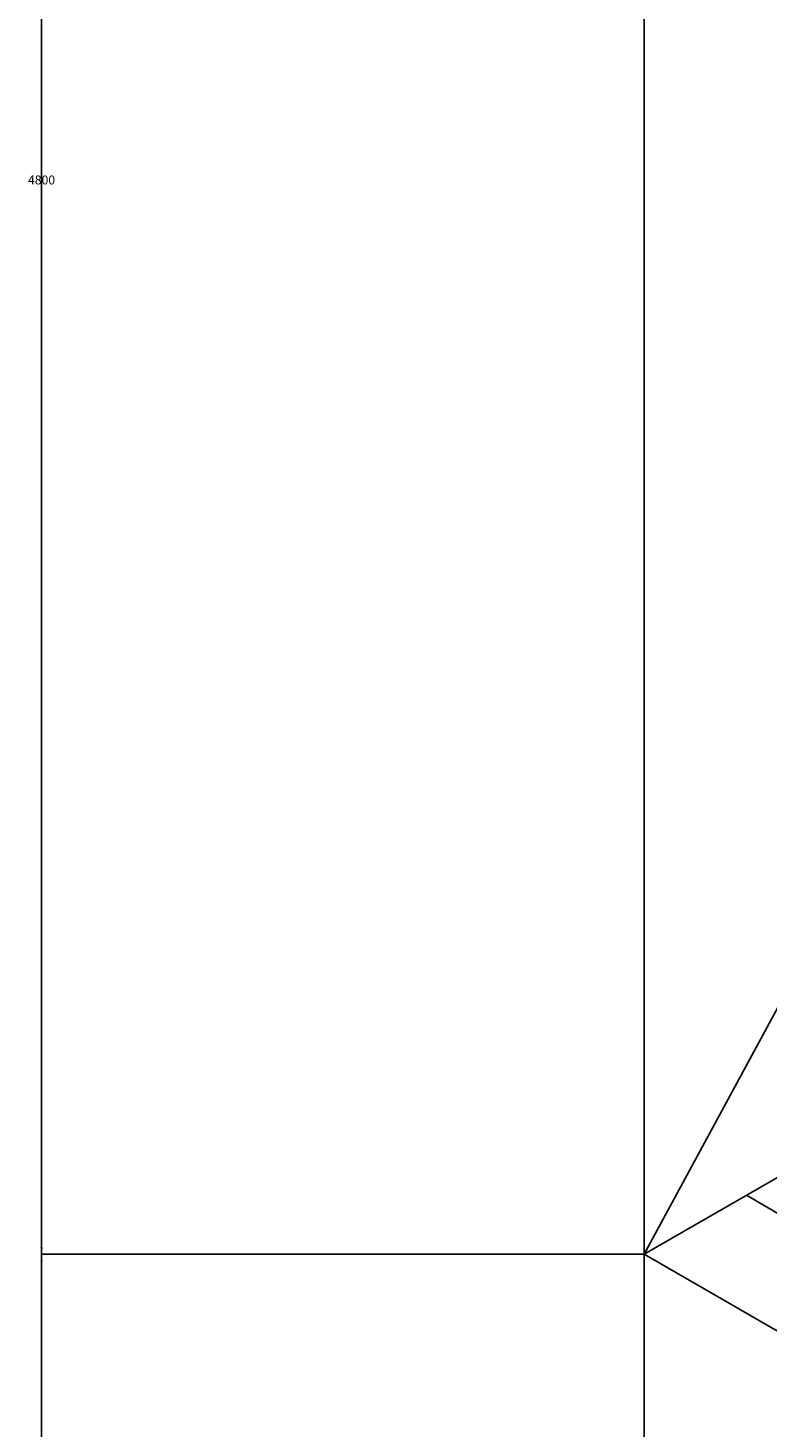
# Model space of a CAD drawing. Units: metres. Extents: x -2391 to 4922, y -635 to 4845.
# Tile 12 of 37: x -2391 to -1978, y 1408 to 2190. Entities that reach past the tile are written whole.
import ezdxf

# ---------------------------------------------------------------- set-up
doc = ezdxf.new("R2010")
doc.units = ezdxf.units.M
doc.header["$MEASUREMENT"] = 0
doc.layers.add('A-ANNO-DIMS', color=2, linetype='Continuous', lineweight=18)
doc.layers.add('A-FLOR-FIXT', color=3, linetype='Continuous', lineweight=25)
doc.styles.get("Standard").update_dxf_attribs({"font": 'arial.ttf'})
doc.dimstyles.get("Standard").update_dxf_attribs({"dimtxt": 5, "dimasz": 4, "dimexe": 0.18, "dimexo": 0.0625, "dimgap": 0.09, "dimtad": 0, "dimtih": 1, "dimtoh": 1, "dimdec": 0, "dimzin": 0, "dimdsep": 46, "dimtxsty": 'Standard', "dimcen": 0.09, "dimadec": 0, "dimazin": 0, "dimtfac": 1, "dimtdec": 0, "dimtofl": 0, "dimtmove": 0, "dimatfit": 3, "dimfxl": 1, "dimtolj": 1, "dimtzin": 0, "dimarcsym": 0})

# ---------------------------------------------------------------- blocks, each defined once
blk = doc.blocks.new('*D8')
at = {"layer": 'A-ANNO-DIMS', "color": 0, "lineweight": -2, "transparency": 16777216}
for p, q in [((-2047.33, 3005.21), (-2047.33, -631.4)), ((4577.76, 2350.21), (4577.76, -631.4)), ((-2043.33, -631.22), (1257.62, -631.22)), ((4573.76, -631.22), (1272.8, -631.22))]:
    blk.add_line(p, q, dxfattribs=at)
at = {"layer": 'A-ANNO-DIMS', "color": 0, "transparency": 16777216}
for points in [[(-2043.33, -630.56), (-2043.33, -631.89), (-2047.33, -631.22)], [(4573.76, -630.56), (4573.76, -631.89), (4577.76, -631.22)]]:
    blk.add_solid(points, dxfattribs=at)
at = {"layer": 'Defpoints', "color": 0, "transparency": 16777216}
for p in [(-2047.33, 3005.28), (4577.76, 2350.28), (4577.76, -631.22)]:
    blk.add_point(p, dxfattribs=at)
at = {"layer": 'A-ANNO-DIMS', "color": 0, "transparency": 16777216, "insert": (1265.21, -631.22), "char_height": 5, "attachment_point": 5}
blk.add_mtext('\\A1;6625', dxfattribs=at)
blk = doc.blocks.new('*D10')
at = {"layer": 'A-ANNO-DIMS', "color": 0, "lineweight": -2, "transparency": 16777216}
for p, q in [((550.68, 4505.28), (-2384.01, 4505.28)), ((-2383.83, 4501.28), (-2383.83, 2107.92)), ((-2383.83, -290.72), (-2383.83, 2102.63)), ((-488.55, -294.72), (-2384.01, -294.72))]:
    blk.add_line(p, q, dxfattribs=at)
at = {"layer": 'A-ANNO-DIMS', "color": 0, "transparency": 16777216}
for points in [[(-2384.5, 4501.28), (-2383.17, 4501.28), (-2383.83, 4505.28)], [(-2384.5, -290.72), (-2383.17, -290.72), (-2383.83, -294.72)]]:
    blk.add_solid(points, dxfattribs=at)
at = {"layer": 'Defpoints', "color": 0, "transparency": 16777216}
for p in [(-2383.83, 4505.28), (550.74, 4505.28), (-488.49, -294.72)]:
    blk.add_point(p, dxfattribs=at)
at = {"layer": 'A-ANNO-DIMS', "color": 0, "transparency": 16777216, "insert": (-2383.83, 2105.28), "char_height": 5, "attachment_point": 5}
blk.add_mtext('\\A1;4800', dxfattribs=at)
blk = doc.blocks.new('*D41')
at = {"layer": 'A-ANNO-DIMS', "color": 0, "lineweight": -2, "transparency": 16777216}
for p, q in [((-2047.3, 3005.33), (-1878.99, 3296.85)), ((-1875.62, 3294.69), (-1104.24, 2849.34)), ((-323.7, 2398.69), (-1095.08, 2844.05)), ((-488.46, 2105.33), (-320.15, 2396.85))]:
    blk.add_line(p, q, dxfattribs=at)
at = {"layer": 'A-ANNO-DIMS', "color": 0, "transparency": 16777216}
for points in [[(-1875.29, 3295.27), (-1875.95, 3294.12), (-1879.08, 3296.69)], [(-323.37, 2399.27), (-324.04, 2398.12), (-320.24, 2396.69)]]:
    blk.add_solid(points, dxfattribs=at)
at = {"layer": 'Defpoints', "color": 0, "transparency": 16777216}
for p in [(-2047.33, 3005.28), (-320.24, 2396.69), (-488.49, 2105.28)]:
    blk.add_point(p, dxfattribs=at)
at = {"layer": 'A-ANNO-DIMS', "color": 0, "transparency": 16777216, "insert": (-1099.66, 2846.69), "char_height": 5, "attachment_point": 5}
blk.add_mtext('\\A1;1800', dxfattribs=at)
blk = doc.blocks.new('*D43')
at = {"layer": 'A-ANNO-DIMS', "color": 0, "lineweight": -2, "transparency": 16777216}
for p, q in [((-2047.4, 2925.28), (-2384.01, 2925.28)), ((-2383.83, 2921.28), (-2383.83, 2217.92)), ((-2383.83, 1509.28), (-2383.83, 2212.63)), ((-2047.4, 1505.28), (-2384.01, 1505.28))]:
    blk.add_line(p, q, dxfattribs=at)
at = {"layer": 'A-ANNO-DIMS', "color": 0, "transparency": 16777216}
for points in [[(-2384.5, 2921.28), (-2383.17, 2921.28), (-2383.83, 2925.28)], [(-2384.5, 1509.28), (-2383.17, 1509.28), (-2383.83, 1505.28)]]:
    blk.add_solid(points, dxfattribs=at)
at = {"layer": 'Defpoints', "color": 0, "transparency": 16777216}
for p in [(-2047.33, 2925.28), (-2383.83, 1505.28), (-2047.33, 1505.28)]:
    blk.add_point(p, dxfattribs=at)
at = {"layer": 'A-ANNO-DIMS', "color": 0, "transparency": 16777216, "insert": (-2383.83, 2215.28), "char_height": 5, "attachment_point": 5}
blk.add_mtext('\\A1;1420', dxfattribs=at)
blk = doc.blocks.new('*D44')
at = {"layer": 'A-ANNO-DIMS', "color": 0, "lineweight": -2, "transparency": 16777216}
for p, q in [((-2047.4, 1505.28), (-2384.01, 1505.28)), ((-2383.83, 1501.28), (-2383.83, 1057.92)), ((-2383.83, 609.28), (-2383.83, 1052.63)), ((-2047.4, 605.28), (-2384.01, 605.28))]:
    blk.add_line(p, q, dxfattribs=at)
at = {"layer": 'A-ANNO-DIMS', "color": 0, "transparency": 16777216}
for points in [[(-2384.5, 1501.28), (-2383.17, 1501.28), (-2383.83, 1505.28)], [(-2384.5, 609.28), (-2383.17, 609.28), (-2383.83, 605.28)]]:
    blk.add_solid(points, dxfattribs=at)
at = {"layer": 'Defpoints', "color": 0, "transparency": 16777216}
for p in [(-2047.33, 1505.28), (-2383.83, 605.28), (-2047.33, 605.28)]:
    blk.add_point(p, dxfattribs=at)
at = {"layer": 'A-ANNO-DIMS', "color": 0, "transparency": 16777216, "insert": (-2383.83, 1055.28), "char_height": 5, "attachment_point": 5}
blk.add_mtext('\\A1;900', dxfattribs=at)
blk = doc.blocks.new('*D46')
at = {"layer": 'A-ANNO-DIMS', "color": 0, "lineweight": -2, "transparency": 16777216}
for p, q in [((-2047.3, 1505.33), (-1887.13, 1801.4)), ((-1883.7, 1799.34), (-1087.36, 1368.5)), ((-281.24, 932.38), (-1077.58, 1363.21)), ((-437.81, 634.57), (-277.64, 930.64))]:
    blk.add_line(p, q, dxfattribs=at)
at = {"layer": 'A-ANNO-DIMS', "color": 0, "transparency": 16777216}
for points in [[(-1883.38, 1799.92), (-1884.01, 1798.75), (-1887.21, 1801.24)], [(-280.92, 932.97), (-281.56, 931.8), (-277.72, 930.48)]]:
    blk.add_solid(points, dxfattribs=at)
at = {"layer": 'Defpoints', "color": 0, "transparency": 16777216}
for p in [(-2047.33, 1505.28), (-277.72, 930.48), (-437.84, 634.52)]:
    blk.add_point(p, dxfattribs=at)
at = {"layer": 'A-ANNO-DIMS', "color": 0, "transparency": 16777216, "insert": (-1082.47, 1365.86), "char_height": 5, "attachment_point": 5}
blk.add_mtext('\\A1;1830', dxfattribs=at)

msp = doc.modelspace()

# ---------------------------------------------------------------- linework, layer by layer
at = {"layer": 'A-FLOR-FIXT'}
for p, q in [((-2047.3343, 1505.2763), (-2047.3343, 3005.2763)), ((-2047.3343, 1505.2763), (-1527.7191, 1805.2763)), ((-1990.2207, 1538.2508), (-1872.4955, 1469.7159)), ((-2047.3343, 1505.2763), (-2047.3343, 605.2763)), ((-1902.9302, 1421.9045), (-2047.3343, 1505.2763))]:
    msp.add_line(p, q, dxfattribs=at)

# ---------------------------------------------------------------- dimensions: what is measured, and where the dimension line sits
at = {"layer": 'A-ANNO-DIMS'}
for base, p1, p2, angle, picture, middle in [((-2383.8343, 4505.2763), (-488.4886, -294.7237), (550.7419, 4505.2763), 90, '*D10', (-2383.8343, 2105.2763)), ((-320.2386, 2396.6938), (-2047.3343, 3005.2763), (-488.4886, 2105.2763), 330, '*D41', (-1099.6615, 2846.6938)), ((-2383.8343, 1505.2763), (-2047.3343, 2925.2763), (-2047.3343, 1505.2763), 90, '*D43', (-2383.8343, 2215.2763)), ((-277.7211, 930.4802), (-2047.3343, 1505.2763), (-437.841, 634.5176), 331.5859855, '*D46', (-1082.4677, 1365.8595)), ((-2383.8343, 605.2763), (-2047.3343, 1505.2763), (-2047.3343, 605.2763), 90, '*D44', (-2383.8343, 1055.2763))]:
    dim = msp.add_linear_dim(base=base, p1=p1, p2=p2, angle=angle, dimstyle='Standard', override={"dimdec": 0, "dimlfac": 1, "dimrnd": 0, "dimzin": 0, "dimdsep": 46, "dimlunit": 2}, dxfattribs=at)
    dim.commit()
    dim.dimension.update_dxf_attribs({"geometry": picture, "text_midpoint": middle})
dim = msp.add_linear_dim(base=(4577.76, -631.2237), p1=(-2047.3343, 3005.2763), p2=(4577.76, 2350.2763), dimstyle='Standard', override={"dimdec": 0, "dimlfac": 1, "dimrnd": 0, "dimzin": 0, "dimdsep": 46, "dimlunit": 2}, dxfattribs=at)
dim.commit()
dim.dimension.update_dxf_attribs({"geometry": '*D8', "text_midpoint": (1265.2128, -631.2237)})

doc.saveas('drawing.dxf')
